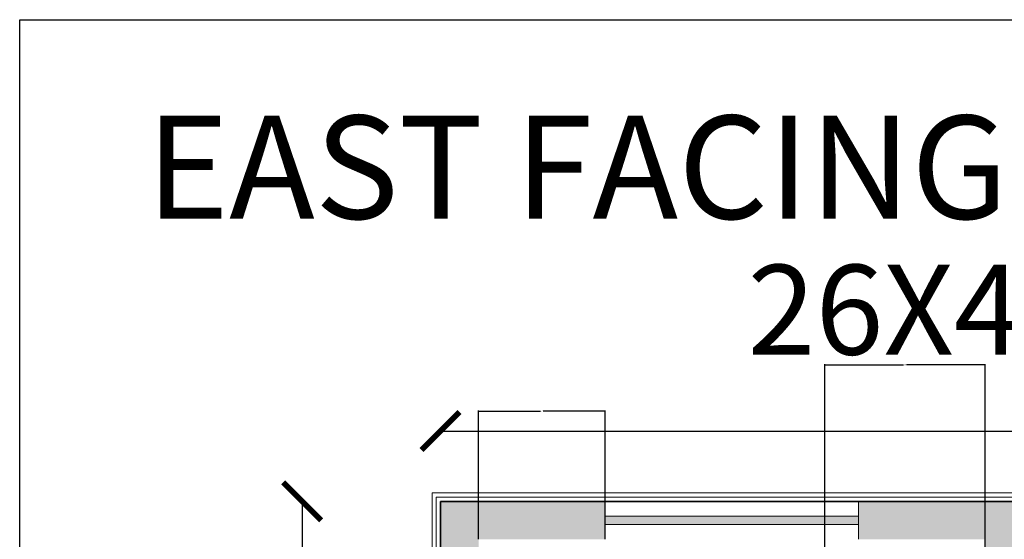
# Model space of a CAD drawing. Units: inches. Extents: x 311 to 815, y -527 to 136.
# Tile 20 of 21: x 311 to 544, y 13 to 136. Entities that reach past the tile are written whole.
import ezdxf

# ---------------------------------------------------------------- set-up
doc = ezdxf.new("R2010")
doc.units = ezdxf.units.IN
doc.header["$MEASUREMENT"] = 0
for name, color, linetype, lineweight in [('A-ANNO-DIMS', 1, 'Continuous', 18), ('A-ANNO-TEXT', 8, 'Continuous', 25), ('A-ANNO-TTLB', 1, 'Continuous', 25), ('A-FLOR-EDGE', 1, 'Continuous', 18), ('A-GLAZ-PATT', 5, 'Continuous', 13), ('A-WALL-PATT', 242, 'Continuous', 13), ('wall', 1, 'Continuous', 35), ('win', 5, 'Continuous', 18)]:
    doc.layers.add(name, color=color, linetype=linetype, lineweight=lineweight)
doc.styles.get("Standard").update_dxf_attribs({"font": 'arial.ttf'})
doc.dimstyles.get("Standard").update_dxf_attribs({"dimtxt": 0.18, "dimasz": 0.18, "dimexe": 0.18, "dimexo": 0.0625, "dimgap": 0.09, "dimtad": 0, "dimtih": 1, "dimtoh": 1, "dimdec": 1, "dimzin": 0, "dimdsep": 46, "dimlunit": 4, "dimtxsty": 'Standard', "dimcen": 0.09, "dimadec": 0, "dimazin": 0, "dimtfac": 1, "dimtdec": 1, "dimtofl": 0, "dimtmove": 0, "dimatfit": 3, "dimfxl": 1, "dimtolj": 1, "dimtzin": 0, "dimarcsym": 0})

# ---------------------------------------------------------------- blocks, each defined once
blk = doc.blocks.new('_ArchTick')
at = {"color": 0, "linetype": 'ByBlock', "const_width": 0.15}
blk.add_lwpolyline([(-0.5, -0.5), (0.5, 0.5)], dxfattribs=at)
blk = doc.blocks.new('_Oblique')
at = {"color": 0, "linetype": 'ByBlock', "lineweight": -2}
blk.add_line((-0.5, -0.5), (0.5, 0.5), dxfattribs=at)
blk = doc.blocks.new('*D2')
at = {"layer": 'A-ANNO-DIMS', "color": 0, "lineweight": -2, "transparency": 16777216}
for p, q in [((410.32, 38.54), (554.61, 38.54)), ((722.32, 38.54), (578.04, 38.54))]:
    blk.add_line(p, q, dxfattribs=at)
at = {"layer": 'Defpoints', "color": 0, "transparency": 16777216}
for p in [(722.32, 38.54), (410.32, 21.87), (722.32, 21.87)]:
    blk.add_point(p, dxfattribs=at)
at = {"layer": 'A-ANNO-DIMS', "color": 0, "lineweight": -2, "transparency": 16777216, "xscale": 9, "yscale": 9, "zscale": 9, "rotation": 180}
blk.add_blockref('_ArchTick', (410.32, 38.54), dxfattribs=at)
at = {"layer": 'A-ANNO-DIMS', "color": 0, "lineweight": -2, "transparency": 16777216, "xscale": 9, "yscale": 9, "zscale": 9}
blk.add_blockref('_Oblique', (722.32, 38.54), dxfattribs=at)
at = {"layer": 'A-ANNO-DIMS', "color": 0, "transparency": 16777216, "insert": (566.32, 38.54), "char_height": 9, "attachment_point": 5}
blk.add_mtext("\\A1;26'", dxfattribs=at)
blk = doc.blocks.new('*D3')
at = {"layer": 'A-ANNO-DIMS', "color": 0, "lineweight": -2, "transparency": 16777216}
for p, q in [((377.54, 21.87), (377.54, -221.61)), ((377.54, -482.13), (377.54, -238.65))]:
    blk.add_line(p, q, dxfattribs=at)
at = {"layer": 'Defpoints', "color": 0, "transparency": 16777216}
for p in [(410.32, 21.87), (377.54, -482.13), (410.32, -482.13)]:
    blk.add_point(p, dxfattribs=at)
at = {"layer": 'A-ANNO-DIMS', "color": 0, "lineweight": -2, "transparency": 16777216, "xscale": 9, "yscale": 9, "zscale": 9}
for name, p, rotation in [('_ArchTick', (377.54, 21.87), 90), ('_Oblique', (377.54, -482.13), 270)]:
    blk.add_blockref(name, p, dxfattribs=dict(at, rotation=rotation))
at = {"layer": 'A-ANNO-DIMS', "color": 0, "transparency": 16777216, "insert": (377.54, -230.13), "char_height": 9, "attachment_point": 5}
blk.add_mtext("\\A1;42'", dxfattribs=at)
blk = doc.blocks.new('WIN-60IN')
for p, q in [((9, 60), (0, 60)), ((3.5, 0), (3.5, 60)), ((5.5, 0), (5.5, 60)), ((9, 0), (0, 0))]:
    blk.add_line(p, q)
blk = doc.blocks.new('*D45')
at = {"layer": 'A-ANNO-DIMS', "color": 0, "lineweight": -2, "transparency": 16777216}
for p, q in [((419.32, 12.93), (419.32, 43.4)), ((419.5, 43.22), (433.99, 43.22)), ((449.14, 43.22), (434.65, 43.22)), ((449.32, 12.93), (449.32, 43.4))]:
    blk.add_line(p, q, dxfattribs=at)
at = {"layer": 'A-ANNO-DIMS', "color": 0, "transparency": 16777216}
for points in [[(419.5, 43.25), (419.5, 43.19), (419.32, 43.22)], [(449.14, 43.25), (449.14, 43.19), (449.32, 43.22)]]:
    blk.add_solid(points, dxfattribs=at)
at = {"layer": 'Defpoints', "color": 0, "transparency": 16777216}
for p in [(449.32, 43.22), (419.32, 12.87), (449.32, 12.87)]:
    blk.add_point(p, dxfattribs=at)
at = {"layer": 'A-ANNO-DIMS', "color": 0, "transparency": 16777216, "insert": (434.32, 43.22), "char_height": 0.18, "attachment_point": 5}
blk.add_mtext('\\A1;2\'-6"', dxfattribs=at)
blk = doc.blocks.new('*D51')
at = {"layer": 'A-ANNO-DIMS', "color": 0, "lineweight": -2, "transparency": 16777216}
for p, q in [((501.32, -103.07), (501.32, 54.4)), ((501.5, 54.22), (519.99, 54.22)), ((539.14, 54.22), (520.65, 54.22)), ((539.32, -112.07), (539.32, 54.4))]:
    blk.add_line(p, q, dxfattribs=at)
at = {"layer": 'A-ANNO-DIMS', "color": 0, "transparency": 16777216}
for points in [[(501.5, 54.25), (501.5, 54.19), (501.32, 54.22)], [(539.14, 54.25), (539.14, 54.19), (539.32, 54.22)]]:
    blk.add_solid(points, dxfattribs=at)
at = {"layer": 'Defpoints', "color": 0, "transparency": 16777216}
for p in [(501.32, 54.22), (501.32, -103.13), (539.32, -112.13)]:
    blk.add_point(p, dxfattribs=at)
at = {"layer": 'A-ANNO-DIMS', "color": 0, "transparency": 16777216, "insert": (520.32, 54.22), "char_height": 0.18, "attachment_point": 5}
blk.add_mtext('\\A1;3\'-2"', dxfattribs=at)

msp = doc.modelspace()

# ---------------------------------------------------------------- hatches: boundary and pattern name
at = {"layer": 'A-GLAZ-PATT'}
h = msp.add_hatch(color=256, dxfattribs=at)
h.dxf.hatch_style = 1
h.paths.add_polyline_path([(415.82, -202.13), (413.82, -202.13), (413.82, -262.13), (415.82, -262.13)])
h.paths.add_polyline_path([(415.82, -390.84), (413.82, -390.84), (413.82, -450.84), (415.82, -450.84)])
h.paths.add_polyline_path([(415.82, -311.57), (413.82, -311.57), (413.82, -335.57), (415.82, -335.57)])
h.paths.add_polyline_path([(509.32, -476.63), (449.32, -476.63), (449.32, -478.63), (509.32, -478.63)])
h.paths.add_polyline_path([(606.82, -476.63), (582.82, -476.63), (582.82, -478.63), (606.82, -478.63)])
h.paths.add_polyline_path([(678.82, -476.63), (654.82, -476.63), (654.82, -478.63), (678.82, -478.63)])
h.paths.add_polyline_path([(718.82, -385.13), (716.82, -385.13), (716.82, -445.13), (718.82, -445.13)])
h.paths.add_polyline_path([(718.82, -262.63), (716.82, -262.63), (716.82, -322.63), (718.82, -322.63)])
h.paths.add_polyline_path([(718.82, -140.13), (716.82, -140.13), (716.82, -200.13), (718.82, -200.13)])
h.paths.add_polyline_path([(718.82, -18.13), (716.82, -18.13), (716.82, -42.13), (718.82, -42.13)])
h.paths.add_polyline_path([(686.82, 18.37), (626.82, 18.37), (626.82, 16.37), (686.82, 16.37)])
h.paths.add_polyline_path([(581.82, 18.37), (557.82, 18.37), (557.82, 16.37), (581.82, 16.37)])
h.paths.add_polyline_path([(509.32, 18.37), (449.32, 18.37), (449.32, 16.37), (509.32, 16.37)])
at = {"layer": 'A-WALL-PATT'}
h = msp.add_hatch(color=256, dxfattribs=at)
h.dxf.hatch_style = 1
h.paths.add_polyline_path([(557.82, 21.87), (509.32, 21.87), (509.32, 12.87), (539.32, 12.87), (539.32, -112.13), (548.32, -112.13), (548.32, -58.63), (557.82, -58.63), (557.82, -49.63), (548.32, -49.63), (548.32, 12.87), (557.82, 12.87)])
h.paths.add_polyline_path([(449.32, 21.87), (410.32, 21.87), (410.32, -15.13), (419.32, -15.13), (419.32, 12.87), (449.32, 12.87)])
h.paths.add_polyline_path([(626.82, 21.87), (581.82, 21.87), (581.82, 12.87), (591.32, 12.87), (591.32, -49.63), (581.82, -49.63), (581.82, -58.63), (591.32, -58.63), (591.32, -112.13), (600.32, -112.13), (600.32, 12.87), (626.82, 12.87)])
h.paths.add_polyline_path([(722.32, 21.87), (686.82, 21.87), (686.82, 12.87), (713.32, 12.87), (713.32, -18.13), (722.32, -18.13)])
h.paths.add_polyline_path([(722.32, -42.13), (713.32, -42.13), (713.32, -73.13), (722.32, -73.13)])
h.paths.add_polyline_path([(501.32, -103.13), (419.32, -103.13), (419.32, -75.13), (410.32, -75.13), (410.32, -126.63), (419.32, -126.63), (419.32, -112.13), (492.32, -112.13), (492.32, -143.13), (501.32, -143.13)])
h.paths.add_polyline_path([(548.32, -165.13), (419.32, -165.13), (419.32, -150.63), (410.32, -150.63), (410.32, -202.13), (419.32, -202.13), (419.32, -174.13), (548.32, -174.13)])
h.paths.add_polyline_path([(722.32, -103.13), (636.32, -103.13), (636.32, -112.13), (713.32, -112.13), (713.32, -140.13), (722.32, -140.13)])
h.paths.add_polyline_path([(548.32, -210.13), (539.32, -210.13), (539.32, -290.13), (419.32, -290.13), (419.32, -262.13), (410.32, -262.13), (410.32, -311.57), (419.32, -311.57), (419.32, -299.13), (469.32, -299.13), (469.32, -348.13), (443.32, -348.13), (443.32, -357.13), (478.32, -357.13), (478.32, -299.13), (548.32, -299.13)])
h.paths.add_polyline_path([(722.32, -200.13), (713.32, -200.13), (713.32, -228.13), (609.32, -228.13), (609.32, -237.13), (713.32, -237.13), (713.32, -262.63), (722.32, -262.63)])
h.paths.add_polyline_path([(722.32, -322.63), (713.32, -322.63), (713.32, -348.13), (633.32, -348.13), (633.32, -357.13), (713.32, -357.13), (713.32, -385.13), (722.32, -385.13)])
h.paths.add_polyline_path([(419.32, -335.57), (410.32, -335.57), (410.32, -390.84), (419.32, -390.84)])
h.paths.add_polyline_path([(419.32, -450.84), (410.32, -450.84), (410.32, -482.13), (449.32, -482.13), (449.32, -473.13), (419.32, -473.13)])
h.paths.add_polyline_path([(582.82, -473.13), (548.32, -473.13), (548.32, -348.13), (539.32, -348.13), (539.32, -473.13), (509.32, -473.13), (509.32, -482.13), (582.82, -482.13)])
h.paths.add_polyline_path([(722.32, -445.13), (713.32, -445.13), (713.32, -473.13), (678.82, -473.13), (678.82, -482.13), (722.32, -482.13)])

# ---------------------------------------------------------------- linework, layer by layer
at = {"layer": 'A-ANNO-TTLB'}
msp.add_lwpolyline([(310.67, 136.01), (815.43, 136.01), (815.43, -506.97), (310.67, -506.97)], close=True, dxfattribs=at)
at = {"layer": 'A-FLOR-EDGE'}
for p, q in [((408.32, -484.13), (408.32, 23.87)), ((724.32, 23.87), (408.32, 23.87)), ((409.32, -483.13), (409.32, 22.87)), ((723.32, 22.87), (409.32, 22.87))]:
    msp.add_line(p, q, dxfattribs=at)
at = {"layer": 'wall'}
for p in [(410.32, -482.13), (722.32, 21.87)]:
    msp.add_line(p, (410.32, 21.87), dxfattribs=at)

# ---------------------------------------------------------------- block references
at = {"layer": 'win', "rotation": 89.99999999999996}
msp.add_blockref('WIN-60IN', (509.32, 12.87), dxfattribs=at)

# ---------------------------------------------------------------- texts
at = {"layer": 'A-ANNO-TEXT', "attachment_point": 1}
for s, width, gutter_width, insert, char_height in [('EAST FACING HOUSE PLAN ', 457.2415, 4.08, (340.62, 113.27), 24.4528), ('26X42 FEET', 176.1888, 3.55, (483, 77.92), 21.281)]:
    msp.add_mtext_dynamic_manual_height_columns(s, width=width, gutter_width=gutter_width, heights=[0], dxfattribs=dict(at, insert=insert, char_height=char_height))

# ---------------------------------------------------------------- dimensions: what is measured, and where the dimension line sits
at = {"layer": 'A-ANNO-DIMS'}
for base, p1, p2, override, picture, middle in [((501.32, 54.22), (539.32, -112.13), (501.32, -103.13), {"dimdec": 1, "dimlfac": 1, "dimrnd": 0, "dimzin": 1, "dimdsep": 46, "dimlunit": 4, "dimfrac": 2}, '*D51', (520.32, 54.22)), ((722.32, 38.54), (410.32, 21.87), (722.32, 21.87), {"dimtxt": 9, "dimasz": 9, "dimgap": 4, "dimblk1": 'ArchTick', "dimblk2": 'Oblique', "dimsah": 1, "dimse1": 1, "dimse2": 1, "dimclrd": 0, "dimclre": 0, "dimclrt": 0}, '*D2', (566.32, 38.54))]:
    dim = msp.add_linear_dim(base=base, p1=p1, p2=p2, dimstyle='Standard', override=override, dxfattribs=at)
    dim.commit()
    dim.dimension.update_dxf_attribs({"geometry": picture, "text_midpoint": middle})
for base, p1, p2, angle, override, picture, middle in [((449.32, 43.22), (419.32, 12.87), (449.32, 12.87), 0, {"dimdec": 1, "dimlfac": 1, "dimrnd": 0, "dimzin": 1, "dimdsep": 46, "dimlunit": 4, "dimfrac": 2}, '*D45', (434.32, 43.22)), ((377.54, -482.13), (410.32, 21.87), (410.32, -482.13), 90, {"dimtxt": 9, "dimasz": 9, "dimgap": 4, "dimblk1": 'ArchTick', "dimblk2": 'Oblique', "dimsah": 1, "dimse1": 1, "dimse2": 1, "dimclrd": 0, "dimclre": 0, "dimclrt": 0}, '*D3', (377.54, -230.13))]:
    dim = msp.add_linear_dim(base=base, p1=p1, p2=p2, angle=angle, dimstyle='Standard', override=override, dxfattribs=at)
    dim.commit()
    dim.dimension.update_dxf_attribs({"geometry": picture, "text_midpoint": middle})

doc.saveas('drawing.dxf')
